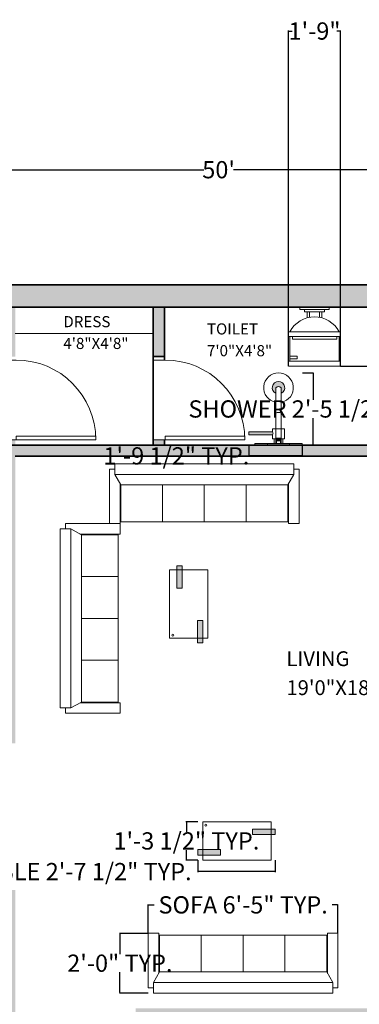
# Model space of a CAD drawing. Units: inches. Extents: x 1319 to 2030, y 219 to 1069.
# Tile 26 of 28: x 1589 to 1727, y 663 to 1063. Entities that reach past the tile are written whole.
import ezdxf

# ---------------------------------------------------------------- set-up
doc = ezdxf.new("R2010")
doc.units = ezdxf.units.IN
doc.header["$MEASUREMENT"] = 0
doc.layers.get('0').update_dxf_attribs({"color": 12})
for name, color, linetype, lineweight in [('A-ANNO-DIMS', 2, 'Continuous', 18), ('A-AREA-IDEN', 250, 'Continuous', 18), ('A-WALL-PATT', 252, 'Continuous', 13), ('C-PROP', 7, 'Continuous', 35), ('closet', 252, 'Continuous', 18), ('doors', 252, 'Continuous', 18), ('furniture', 250, 'Continuous', 18), ('PLUMBING FIXTURES', 252, 'Continuous', 18), ('walls', 250, 'Continuous', 35)]:
    doc.layers.add(name, color=color, linetype=linetype, lineweight=lineweight)
doc.styles.get("Standard").update_dxf_attribs({"font": 'arial.ttf'})
doc.dimstyles.get("Standard").update_dxf_attribs({"dimtxt": 7, "dimasz": 0.18, "dimexe": 0.18, "dimexo": 0.0625, "dimgap": 0.09, "dimtad": 0, "dimtih": 1, "dimtoh": 1, "dimzin": 0, "dimdsep": 46, "dimlunit": 3, "dimtxsty": 'Standard', "dimcen": 0.09, "dimadec": 0, "dimazin": 0, "dimtfac": 1, "dimtofl": 0, "dimtmove": 0, "dimatfit": 3, "dimfxl": 1, "dimtolj": 1, "dimtzin": 0, "dimarcsym": 0})

# ---------------------------------------------------------------- blocks, each defined once
blk = doc.blocks.new('*U2')
for p, q in [((0, 0), (0, -6)), ((40, 0), (40, -6))]:
    blk.add_line(p, q)
blk.add_lwpolyline([(0, 0), (0, 40), (1.75, 40), (1.75, 0)], close=True)
blk.add_arc((0, 0), 40, 0, 90)
blk = doc.blocks.new('FABRIC SOFA 4S')
at = {"layer": 'furniture'}
for p, q in [((0, -51), (0, 51)), ((6, 51), (0, 51)), ((3, 54), (34, 54)), ((3, 51), (3, 54)), ((6, -51), (6, 51)), ((12, 47.63), (6, 51)), ((34, 48), (34, 54)), ((11.14, 48), (34, 48)), ((33, 23.81), (12, 23.81)), ((33, 0), (12, 0)), ((33, -23.81), (12, -23.81)), ((6, -51), (12, -47.63)), ((11.54, -48), (34, -48)), ((34, -48), (34, -54)), ((6, -51), (0, -51)), ((3, -54), (3, -51)), ((3, -54), (34, -54))]:
    blk.add_line(p, q, dxfattribs=at)
blk.add_lwpolyline([(12, -47.63), (12, 47.63), (33, 47.63), (33, -47.63)], close=True, dxfattribs=at)
blk = doc.blocks.new('*U25')
for p, q in [((-10, 22), (-10, 12)), ((-10, 21), (-7, 21)), ((-7, 20), (-10, 20)), ((-7, 21), (-7, 20)), ((10, 12), (10, 22)), ((10.5, 12), (-10.5, 12)), ((-10.5, 10), (-10.5, 12)), ((9, 13), (-9, 13)), ((-9, 13), (-9, 12)), ((9, 12), (9, 13)), ((10.5, 12), (10.5, 10)), ((10.5, 10), (-10.5, 10)), ((-3, 4.4065), (-3, 2)), ((-2, 2), (-2, 4.1658)), ((2, 4.1658), (2, 2)), ((3, 2), (3, 4.4065)), ((4, 2), (-4, 2)), ((-4, 2), (-4, 1)), ((4, 1), (4, 2))]:
    blk.add_line(p, q)
for points in [[(10.5, 22), (10.5, 24), (-10.5, 24), (-10.5, 22)], [(6, 0), (6, 1), (-6, 1), (-6, 0)]]:
    blk.add_lwpolyline(points, close=True)
blk.add_arc((0, 15.3333), 11.3333, 208.0725, 331.9275)
blk = doc.blocks.new('O.H SHOWER-PL')
at = {"layer": 'PLUMBING FIXTURES'}
for points in [[(-1.84, 0), (-1.84, -0.25), (1.84, -0.25), (1.84, 0)], [(0.46, -8.72), (0.46, -9.67, -0.422337), (-0.46, -9.67), (-0.46, -8.72, 4.325472)]]:
    blk.add_hatch(color=256, dxfattribs=at).paths.add_polyline_path(points)
for p, q in [((-1.84, 0), (-1.84, -0.25)), ((1.84, 0), (-1.84, 0)), ((1.84, 0), (1.84, -0.25)), ((1.84, -0.25), (-1.84, -0.25)), ((-0.46, -0.25), (-0.46, -9.67)), ((0.46, -0.25), (0.46, -9.67))]:
    blk.add_line(p, q, dxfattribs=at)
for centre, radius, start, end in [((0, -4.48), 1.03, 243.53, 296.47), ((0, -9.67), 2.5, 100.61, 79.39), ((0, -9.67), 1.05, 116.0349, 63.9652), ((0, -9.22), 0.643, 224.2078, 315.7922)]:
    blk.add_arc(centre, radius, start, end, dxfattribs=at)
blk = doc.blocks.new('DIVERTER-PL')
at = {"layer": 'PLUMBING FIXTURES'}
for points in [[(4, 0), (-4, 0), (-4, -0.25), (4, -0.25)], [(0.38, -1.14), (0.38, -0.7), (-0.37, -0.7), (-0.37, -1.14)], [(1, -1.75, 0.30818), (1, -2.25), (5, -2.25), (5, -1.75)]]:
    blk.add_hatch(color=256, dxfattribs=at).paths.add_polyline_path(points)
for p, q in [((-4, 0), (-4, -0.25)), ((-4, 0), (4, 0)), ((4, 0), (4, -0.25)), ((-4, -0.25), (4, -0.25)), ((-4, -0.25), (4, -0.25)), ((-1, -1.05), (-0.37, -1.05)), ((-1, -1.05), (-1, -2.75)), ((-0.75, -0.25), (-0.75, -1.05)), ((-0.37, -0.7), (0.38, -0.7)), ((-0.37, -0.7), (-0.37, -1.14)), ((-0.37, -1.14), (0.38, -1.14)), ((-0.32, -0.7), (-0.32, -0.25)), ((0.32, -0.7), (0.32, -0.25)), ((0.38, -0.7), (0.38, -1.14)), ((0.38, -1.05), (1, -1.05)), ((0.75, -0.25), (0.75, -1.05)), ((1, -1.05), (1, -1.75)), ((-1, -2.75), (1, -2.75)), ((1, -2.25), (1, -2.75))]:
    blk.add_line(p, q, dxfattribs=at)
at = {"layer": 'PLUMBING FIXTURES', "ltscale": 12}
for p, q in [((1, -1.75), (5, -1.75)), ((1, -2.25), (5, -2.25)), ((5, -2.25), (5, -1.75))]:
    blk.add_line(p, q, dxfattribs=at)
at = {"layer": 'PLUMBING FIXTURES'}
blk.add_arc((1.37, -2), 0.444, 145.7435, 214.2565, dxfattribs=at)
blk = doc.blocks.new('A$C7F153053')
at = {"layer": 'PLUMBING FIXTURES', "xscale": -1, "rotation": 270}
for name in ['DIVERTER-PL', 'O.H SHOWER-PL']:
    blk.add_blockref(name, (12.17, 4), dxfattribs=at)
blk = doc.blocks.new('*D28')
at = {"layer": 'A-ANNO-DIMS', "color": 0, "lineweight": -2, "transparency": 16777216}
for p, q in [((1369.84, 1002.94), (1369.84, 1001.77)), ((1969.84, 1002.94), (1969.84, 1001.77)), ((1370.02, 1001.95), (1663.81, 1001.95)), ((1969.66, 1001.95), (1675.87, 1001.95))]:
    blk.add_line(p, q, dxfattribs=at)
at = {"layer": 'A-ANNO-DIMS', "color": 0, "transparency": 16777216}
for points in [[(1370.02, 1001.98), (1370.02, 1001.92), (1369.84, 1001.95)], [(1969.66, 1001.98), (1969.66, 1001.92), (1969.84, 1001.95)]]:
    blk.add_solid(points, dxfattribs=at)
at = {"layer": 'Defpoints', "color": 0, "transparency": 16777216}
for p in [(1369.84, 1003), (1969.84, 1003), (1969.84, 1001.95)]:
    blk.add_point(p, dxfattribs=at)
at = {"layer": 'A-ANNO-DIMS', "color": 0, "transparency": 16777216, "insert": (1669.84, 1001.95), "char_height": 7, "attachment_point": 5}
blk.add_mtext("\\A1;50'", dxfattribs=at)
blk = doc.blocks.new('TABLE-COCKTAIL')
h = blk.add_hatch(color=256)
h.dxf.hatch_style = 1
h.paths.add_polyline_path([(4.23, 29.31), (2.04, 29.31), (2.04, 22.19), (4.23, 22.19)])
h.paths.add_polyline_path([(4.23, 31.28), (2.04, 31.28), (2.04, 29.31), (4.23, 29.31)])
h.paths.add_polyline_path([(12.58, 9.09), (10.39, 9.09), (10.39, 1.62), (12.58, 1.62)])
h.paths.add_polyline_path([(12.58, 1.62), (10.39, 1.62), (10.39, 0), (12.58, 0)])
for p, q in [((0, 29.31), (0, 1.62)), ((15.53, 29.31), (0, 29.31)), ((2.04, 31.28), (4.23, 31.28)), ((2.04, 22.19), (2.04, 31.28)), ((4.23, 31.28), (4.23, 22.19)), ((15.53, 1.62), (15.53, 29.31)), ((4.23, 22.19), (2.04, 22.19)), ((10.39, 9.09), (12.58, 9.09)), ((10.39, 0), (10.39, 9.09)), ((12.58, 9.09), (12.58, 0)), ((0, 1.62), (15.53, 1.62)), ((12.58, 0), (10.39, 0))]:
    blk.add_line(p, q)
blk.add_circle((14.17, 28.1), 0.401)
blk = doc.blocks.new('*D36')
at = {"layer": 'A-ANNO-DIMS', "color": 0, "lineweight": -2, "transparency": 16777216}
for p, q in [((1641.31, 692.19), (1641.31, 703.85)), ((1641.49, 703.67), (1643.72, 703.67)), ((1718.11, 703.67), (1715.88, 703.67)), ((1718.29, 692.19), (1718.29, 703.85))]:
    blk.add_line(p, q, dxfattribs=at)
at = {"layer": 'A-ANNO-DIMS', "color": 0, "transparency": 16777216}
for points in [[(1641.49, 703.7), (1641.49, 703.64), (1641.31, 703.67)], [(1718.11, 703.7), (1718.11, 703.64), (1718.29, 703.67)]]:
    blk.add_solid(points, dxfattribs=at)
at = {"layer": 'Defpoints', "color": 0, "transparency": 16777216}
for p in [(1718.29, 703.67), (1641.31, 692.12), (1718.29, 692.12)]:
    blk.add_point(p, dxfattribs=at)
at = {"layer": 'A-ANNO-DIMS', "color": 0, "transparency": 16777216, "insert": (1679.8, 703.67), "char_height": 7, "attachment_point": 5}
blk.add_mtext('\\A1;SOFA 6\'-5" TYP.', dxfattribs=at)
blk = doc.blocks.new('*D37')
at = {"layer": 'A-ANNO-DIMS', "color": 0, "lineweight": -2, "transparency": 16777216}
for p, q in [((1641.25, 692.12), (1629.59, 692.12)), ((1629.77, 691.94), (1629.77, 683.67)), ((1629.77, 668.07), (1629.77, 676.34)), ((1641.25, 667.89), (1629.59, 667.89))]:
    blk.add_line(p, q, dxfattribs=at)
at = {"layer": 'A-ANNO-DIMS', "color": 0, "transparency": 16777216}
for points in [[(1629.74, 691.94), (1629.8, 691.94), (1629.77, 692.12)], [(1629.74, 668.07), (1629.8, 668.07), (1629.77, 667.89)]]:
    blk.add_solid(points, dxfattribs=at)
at = {"layer": 'Defpoints', "color": 0, "transparency": 16777216}
for p in [(1629.77, 692.12), (1641.31, 692.12), (1641.31, 667.89)]:
    blk.add_point(p, dxfattribs=at)
at = {"layer": 'A-ANNO-DIMS', "color": 0, "transparency": 16777216, "insert": (1629.77, 680.01), "char_height": 7, "attachment_point": 5}
blk.add_mtext('\\A1;2\'-0" TYP.', dxfattribs=at)
blk = doc.blocks.new('*D40')
at = {"layer": 'A-ANNO-DIMS', "color": 0, "lineweight": -2, "transparency": 16777216}
for p, q in [((1703.84, 919.51), (1708.35, 919.51)), ((1708.17, 919.33), (1708.17, 908.58)), ((1708.17, 890.41), (1708.17, 901.15)), ((1703.84, 890.23), (1708.35, 890.23))]:
    blk.add_line(p, q, dxfattribs=at)
at = {"layer": 'A-ANNO-DIMS', "color": 0, "transparency": 16777216}
for points in [[(1708.14, 919.33), (1708.2, 919.33), (1708.17, 919.51)], [(1708.14, 890.41), (1708.2, 890.41), (1708.17, 890.23)]]:
    blk.add_solid(points, dxfattribs=at)
at = {"layer": 'Defpoints', "color": 0, "transparency": 16777216}
for p in [(1703.78, 919.51), (1703.78, 890.23), (1708.17, 890.23)]:
    blk.add_point(p, dxfattribs=at)
at = {"layer": 'A-ANNO-DIMS', "color": 0, "transparency": 16777216, "insert": (1708.17, 904.87), "char_height": 7, "attachment_point": 5}
blk.add_mtext('\\A1;SHOWER 2\'-5 1/2" TYP.', dxfattribs=at)
blk = doc.blocks.new('*D41')
at = {"layer": 'A-ANNO-DIMS', "color": 0, "lineweight": -2, "transparency": 16777216}
for p, q in [((1682.12, 890.16), (1682.12, 885.66)), ((1703.78, 890.16), (1703.78, 885.66)), ((1682.12, 885.84), (1681.94, 885.84)), ((1703.6, 885.84), (1682.3, 885.84))]:
    blk.add_line(p, q, dxfattribs=at)
at = {"layer": 'A-ANNO-DIMS', "color": 0, "transparency": 16777216}
for points in [[(1682.3, 885.87), (1682.3, 885.81), (1682.12, 885.84)], [(1703.6, 885.87), (1703.6, 885.81), (1703.78, 885.84)]]:
    blk.add_solid(points, dxfattribs=at)
at = {"layer": 'Defpoints', "color": 0, "transparency": 16777216}
for p in [(1682.12, 890.23), (1703.78, 890.23), (1682.12, 885.84)]:
    blk.add_point(p, dxfattribs=at)
at = {"layer": 'A-ANNO-DIMS', "color": 0, "transparency": 16777216, "insert": (1652.69, 885.84), "char_height": 7, "attachment_point": 5}
blk.add_mtext('\\A1;1\'-9 1/2" TYP.', dxfattribs=at)
blk = doc.blocks.new('*D44')
at = {"layer": 'A-ANNO-DIMS', "color": 0, "lineweight": -2, "transparency": 16777216}
for p, q in [((1661.46, 721.8), (1661.46, 716.99)), ((1692.74, 721.8), (1692.74, 716.99)), ((1661.46, 717.17), (1661.28, 717.17)), ((1692.56, 717.17), (1661.64, 717.17))]:
    blk.add_line(p, q, dxfattribs=at)
at = {"layer": 'A-ANNO-DIMS', "color": 0, "transparency": 16777216}
for points in [[(1661.64, 717.2), (1661.64, 717.14), (1661.46, 717.17)], [(1692.56, 717.2), (1692.56, 717.14), (1692.74, 717.17)]]:
    blk.add_solid(points, dxfattribs=at)
at = {"layer": 'Defpoints', "color": 0, "transparency": 16777216}
for p in [(1661.46, 721.86), (1692.74, 721.86), (1661.46, 717.17)]:
    blk.add_point(p, dxfattribs=at)
at = {"layer": 'A-ANNO-DIMS', "color": 0, "transparency": 16777216, "insert": (1602.51, 717.17), "char_height": 7, "attachment_point": 5}
blk.add_mtext('\\A1;LOW TABLE 2\'-7 1/2" TYP.', dxfattribs=at)
blk = doc.blocks.new('*D45')
at = {"layer": 'A-ANNO-DIMS', "color": 0, "lineweight": -2, "transparency": 16777216}
for p, q in [((1661.4, 737.38), (1656.59, 737.38)), ((1656.77, 737.2), (1656.77, 733.33)), ((1656.77, 722.04), (1656.77, 725.91)), ((1661.4, 721.86), (1656.59, 721.86))]:
    blk.add_line(p, q, dxfattribs=at)
at = {"layer": 'A-ANNO-DIMS', "color": 0, "transparency": 16777216}
for points in [[(1656.74, 737.2), (1656.8, 737.2), (1656.77, 737.38)], [(1656.74, 722.04), (1656.8, 722.04), (1656.77, 721.86)]]:
    blk.add_solid(points, dxfattribs=at)
at = {"layer": 'Defpoints', "color": 0, "transparency": 16777216}
for p in [(1656.77, 737.38), (1661.46, 737.38), (1661.46, 721.86)]:
    blk.add_point(p, dxfattribs=at)
at = {"layer": 'A-ANNO-DIMS', "color": 0, "transparency": 16777216, "insert": (1656.77, 729.62), "char_height": 7, "attachment_point": 5}
blk.add_mtext('\\A1;1\'-3 1/2" TYP.', dxfattribs=at)
blk = doc.blocks.new('*D70')
at = {"layer": 'A-ANNO-DIMS', "color": 0, "lineweight": -2, "transparency": 16777216}
for p, q in [((1698.27, 922.29), (1698.27, 1058.4)), ((1698.45, 1058.22), (1699.7, 1058.22)), ((1719.09, 1058.22), (1717.83, 1058.22)), ((1719.27, 922.29), (1719.27, 1058.4))]:
    blk.add_line(p, q, dxfattribs=at)
at = {"layer": 'A-ANNO-DIMS', "color": 0, "transparency": 16777216}
for points in [[(1698.45, 1058.25), (1698.45, 1058.19), (1698.27, 1058.22)], [(1719.09, 1058.25), (1719.09, 1058.19), (1719.27, 1058.22)]]:
    blk.add_solid(points, dxfattribs=at)
at = {"layer": 'Defpoints', "color": 0, "transparency": 16777216}
for p in [(1719.27, 1058.22), (1698.27, 922.23), (1719.27, 922.23)]:
    blk.add_point(p, dxfattribs=at)
at = {"layer": 'A-ANNO-DIMS', "color": 0, "transparency": 16777216, "insert": (1708.77, 1058.22), "char_height": 7, "attachment_point": 5}
blk.add_mtext('\\A1;1\'-9"', dxfattribs=at)
blk = doc.blocks.new('*D71')
at = {"layer": 'A-ANNO-DIMS', "color": 0, "lineweight": -2, "transparency": 16777216}
for p, q in [((1714.83, 946.23), (2012.57, 946.23)), ((2012.39, 946.05), (2012.39, 937.89)), ((2012.39, 922.41), (2012.39, 930.56)), ((1719.33, 922.23), (2012.57, 922.23))]:
    blk.add_line(p, q, dxfattribs=at)
at = {"layer": 'A-ANNO-DIMS', "color": 0, "transparency": 16777216}
for points in [[(2012.36, 946.05), (2012.42, 946.05), (2012.39, 946.23)], [(2012.36, 922.41), (2012.42, 922.41), (2012.39, 922.23)]]:
    blk.add_solid(points, dxfattribs=at)
at = {"layer": 'Defpoints', "color": 0, "transparency": 16777216}
for p in [(1714.77, 946.23), (2012.39, 946.23), (1719.27, 922.23)]:
    blk.add_point(p, dxfattribs=at)
at = {"layer": 'A-ANNO-DIMS', "color": 0, "transparency": 16777216, "insert": (2012.39, 934.23), "char_height": 7, "attachment_point": 5}
blk.add_mtext('\\A1;2\'-0"', dxfattribs=at)

msp = doc.modelspace()

# ---------------------------------------------------------------- hatches: boundary and pattern name
at = {"layer": 'A-WALL-PATT'}
h = msp.add_hatch(color=256, dxfattribs=at)
h.dxf.hatch_style = 1
h.paths.add_polyline_path([(1378.843, 946.227), (1960.843, 946.227), (1960.843, 860.616), (1922.194, 860.616), (1922.194, 851.616), (1960.843, 851.616), (1960.843, 304.227), (1578.343, 304.227), (1578.343, 295.227), (1969.843, 295.227), (1969.843, 955.227), (1369.843, 955.227), (1369.843, 295.227), (1378.843, 295.227)])
h = msp.add_hatch(color=256, dxfattribs=at)
h.dxf.hatch_style = 1
h.paths.add_polyline_path([(1856.292, 860.616), (1812.343, 860.616), (1812.343, 851.616), (1812.343, 700.993), (1816.843, 700.993), (1816.843, 851.616), (1856.292, 851.616)])
h.paths.add_polyline_path([(1960.843, 663.616), (1812.343, 663.616), (1782.783, 663.616), (1782.783, 659.116), (1812.343, 659.116), (1960.843, 659.116)])
h.paths.add_polyline_path([(1857.424, 659.116), (1852.924, 659.116), (1852.924, 616.807), (1857.424, 616.807)])
h.paths.add_polyline_path([(1735.843, 661.727), (1731.843, 661.727), (1636.133, 661.727), (1636.133, 657.227), (1731.343, 657.227), (1731.343, 481.227), (1618.616, 481.227), (1618.616, 472.227), (1639.343, 472.227), (1639.343, 384.227), (1627.044, 384.227), (1627.044, 375.227), (1648.343, 375.227), (1648.343, 384.227), (1648.343, 472.227), (1750.706, 472.227), (1750.706, 481.227), (1735.843, 481.227), (1735.843, 657.727)])
h.paths.add_polyline_path([(1587.343, 481.227), (1578.343, 481.227), (1578.343, 375.227), (1597.622, 375.227), (1597.622, 384.227), (1587.343, 384.227)])
h.paths.add_polyline_path([(1769.593, 384.227), (1693.482, 384.227), (1693.482, 375.227), (1769.593, 375.227)])
h.paths.add_polyline_path([(1775.828, 481.227), (1765.831, 481.227), (1765.831, 472.227), (1775.828, 472.227)])
h.paths.add_polyline_path([(1824.625, 481.227), (1820.343, 481.227), (1820.343, 476.727), (1824.625, 476.727), (1824.625, 477.545)], flags=0)
h.paths.add_polyline_path([(1896.843, 481.227), (1852.26, 481.227), (1852.26, 476.727), (1892.343, 476.727), (1892.343, 384.227), (1881.742, 384.227), (1881.742, 375.227), (1913.435, 375.227), (1913.435, 384.227), (1896.843, 384.227)])
h.paths.add_polyline_path([(1960.843, 481.227), (1931.341, 481.227), (1931.341, 476.727), (1960.843, 476.727)])
h.paths.add_polyline_path([(1736.343, 918.227), (1731.843, 918.227), (1731.843, 890.227), (1582.843, 890.227), (1582.843, 781.727), (1582.843, 769.171), (1587.343, 769.171), (1587.343, 781.727), (1587.343, 885.727), (1731.843, 885.727), (1731.843, 851.616), (1736.343, 851.616), (1736.343, 890.227)])
h.paths.add_polyline_path([(1781.022, 860.616), (1773.021, 860.616, -0.0322281), (1773.289, 856.464), (1773.289, 851.616), (1781.022, 851.616)])
h.paths.add_polyline_path([(1587.343, 946.227), (1582.843, 946.227), (1582.843, 926.136), (1587.343, 926.136)])
h.paths.add_polyline_path([(1647.843, 946.227), (1643.343, 946.227), (1643.343, 926.136), (1647.843, 926.136)])
h.paths.add_polyline_path([(1543.343, 786.227), (1429.843, 786.227), (1429.843, 757.555), (1434.343, 757.555), (1438.843, 757.555), (1438.843, 781.727), (1543.343, 781.727)])
h.paths.add_polyline_path([(1543.343, 781.727), (1538.843, 781.727), (1538.843, 709.727), (1534.597, 709.727), (1534.597, 705.227), (1543.343, 705.227), (1543.343, 709.727)])
h.paths.add_polyline_path([(1499.955, 709.727), (1438.843, 709.727), (1438.843, 734.463), (1429.843, 734.463), (1429.843, 552.227), (1470.241, 552.227), (1470.241, 561.227), (1438.843, 561.227), (1438.843, 705.227), (1499.955, 705.227)])
h.paths.add_polyline_path([(1587.343, 709.727), (1582.843, 709.727), (1582.843, 561.227), (1543.433, 561.227), (1543.433, 552.227), (1587.343, 552.227)])
h.paths.add_polyline_path([(1546.835, 709.727), (1543.343, 709.727), (1543.343, 705.227), (1546.835, 705.227)])
h.paths.add_polyline_path([(1582.843, 709.727), (1579.15, 709.727), (1579.15, 705.227), (1582.843, 705.227)], flags=17)
h.paths.add_polyline_path([(1548.368, 786.227), (1543.343, 786.227), (1543.343, 781.727), (1548.368, 781.727)])
h.paths.add_polyline_path([(1582.843, 786.227), (1580.683, 786.227), (1580.683, 781.727), (1582.843, 781.727)])
h.paths.add_polyline_path([(1587.343, 892.402), (1582.843, 892.402), (1582.843, 890.227), (1587.343, 890.227)], flags=17)
h.paths.add_polyline_path([(1647.843, 892.402), (1643.343, 892.402), (1643.343, 890.227), (1647.843, 890.227)], flags=17)
h.paths.add_polyline_path([(1740.974, 856.464), (1740.974, 860.616), (1736.343, 860.616), (1736.343, 851.616), (1740.974, 851.616)])
h.paths.add_polyline_path([(1853.989, 384.227), (1820.343, 384.227), (1820.343, 402.924), (1815.843, 402.924), (1815.843, 375.227), (1853.989, 375.227)])
h.paths.add_polyline_path([(1892.343, 436.227), (1820.343, 436.227), (1820.343, 481.227), (1815.843, 481.227), (1815.843, 431.727), (1892.343, 431.727)])
h.paths.add_polyline_path([(1849.175, 481.227), (1824.625, 481.227), (1824.625, 477.545), (1825.699, 477.545), (1825.699, 453.018, 0.4014527), (1849.175, 477.545)], flags=0)
h.paths.add_polyline_path([(1960.843, 384.227), (1941.188, 384.227), (1941.188, 375.227), (1960.843, 375.227)])
h.paths.add_polyline_path([(1902.267, 481.227), (1896.843, 481.227), (1896.843, 476.727), (1902.267, 476.727), (1902.267, 477.44)], flags=0)

# ---------------------------------------------------------------- linework, layer by layer
at = {"layer": 'C-PROP'}
msp.add_line((1369.843, 955.227), (1969.843, 955.227), dxfattribs=at)
at = {"layer": 'closet'}
msp.add_line((1587.343, 935.472), (1643.343, 935.472), dxfattribs=at)
at = {"layer": 'walls'}
for p, q in [((1378.843, 946.227), (1960.843, 946.227)), ((1643.343, 890.227), (1643.343, 946.227)), ((1647.843, 924.716), (1647.843, 946.227)), ((1643.343, 926.136), (1647.843, 926.136)), ((1647.843, 890.227), (1647.843, 892.402)), ((1582.843, 890.227), (1731.843, 890.227)), ((1587.343, 885.727), (1731.843, 885.727))]:
    msp.add_line(p, q, dxfattribs=at)

# ---------------------------------------------------------------- block references
at = {"layer": 'doors', "xscale": -0.8078659498341503, "yscale": 0.8078659498341503, "zscale": 0.8078659498341503, "rotation": 270}
for p in [(1587.69, 892.402), (1648.19, 892.402)]:
    msp.add_blockref('*U2', p, dxfattribs=at)
at = {"layer": 'furniture', "yscale": 0.7127038693416449, "zscale": 0.7127038693416449, "rotation": 270}
for p, xscale in [((1664.047, 882.622), 0.7127038693416449), ((1679.8, 667.892), -0.7127038693416449)]:
    msp.add_blockref('FABRIC SOFA 4S', p, dxfattribs=dict(at, xscale=xscale))
at = {"layer": 'furniture', "xscale": 0.7127038693416449, "yscale": 0.7127038693416449, "zscale": 0.7127038693416449}
msp.add_blockref('FABRIC SOFA 4S', (1605.606, 819.904), dxfattribs=at)
at = {"layer": 'furniture'}
for p, rotation in [((1665.489, 841.233), 180), ((1692.741, 721.858), 90.00000000000365)]:
    msp.add_blockref('TABLE-COCKTAIL', p, dxfattribs=dict(at, rotation=rotation))
at = {"layer": 'PLUMBING FIXTURES', "xscale": -1, "rotation": 180}
msp.add_blockref('*U25', (1708.765, 946.227), dxfattribs=at)
at = {"layer": 'PLUMBING FIXTURES', "xscale": -2.406230429091579, "yscale": 2.406230429091579, "zscale": 2.406230429091579, "rotation": 90}
msp.add_blockref('A$C7F153053', (1703.778, 919.501), dxfattribs=at)

# ---------------------------------------------------------------- texts
at = {"layer": 'A-AREA-IDEN'}
for s, height, p in [('DRESS', 4.5146, (1606.812, 938.031)), ('TOILET', 4.5146, (1665.108, 935.092)), ('4\'8"X4\'8"', 4.5146, (1606.812, 929.207)), ('7\'0"X4\'8"', 4.5146, (1665.108, 926.268)), ('LIVING', 6.0112, (1697.378, 800.537)), ('19\'0"X18\'8"', 6.01124, (1697.378, 788.788))]:
    msp.add_text(s, height=height, dxfattribs=at).set_placement(p)

# ---------------------------------------------------------------- dimensions: what is measured, and where the dimension line sits
at = {"layer": 'A-ANNO-DIMS'}
for base, p1, p2, override, picture, middle in [((1719.265, 1058.218), (1698.265, 922.227), (1719.265, 922.227), {"dimdec": 1, "dimlfac": 1, "dimrnd": 0, "dimzin": 1, "dimdsep": 46, "dimlunit": 4, "dimfrac": 2}, '*D70', (1708.765, 1058.218)), ((1969.843, 1001.954), (1369.843, 1003), (1969.843, 1003), {"dimclrd": 0, "dimclre": 0, "dimclrt": 0}, '*D28', (1669.843, 1001.954))]:
    dim = msp.add_linear_dim(base=base, p1=p1, p2=p2, dimstyle='Standard', override=override, dxfattribs=at)
    dim.commit()
    dim.dimension.update_dxf_attribs({"geometry": picture, "text_midpoint": middle})
dim = msp.add_linear_dim(base=(2012.394, 946.227), p1=(1719.265, 922.227), p2=(1714.765, 946.227), angle=90, dimstyle='Standard', override={"dimdec": 1, "dimlfac": 1, "dimrnd": 0, "dimzin": 1, "dimdsep": 46, "dimlunit": 4, "dimfrac": 2}, dxfattribs=at)
dim.commit()
dim.dimension.update_dxf_attribs({"geometry": '*D71', "text_midpoint": (2012.394, 934.227)})
for base, p1, p2, angle, text, picture, middle in [((1708.17, 890.227), (1703.778, 919.506), (1703.778, 890.227), 270, 'SHOWER <> TYP.', '*D40', (1708.17, 904.867)), ((1682.122, 885.835), (1703.778, 890.227), (1682.122, 890.227), 180, '<> TYP.', '*D41', (1652.692, 885.835)), ((1661.464, 717.166), (1692.742, 721.858), (1661.464, 721.858), 180, 'LOW TABLE <> TYP.', '*D44', (1602.515, 717.166)), ((1656.772, 737.383), (1661.464, 721.858), (1661.464, 737.383), 90, '<> TYP.', '*D45', (1656.772, 729.62)), ((1629.768, 692.124), (1641.314, 667.892), (1641.314, 692.124), 90, '<> TYP.', '*D37', (1629.768, 680.008))]:
    dim = msp.add_linear_dim(base=base, p1=p1, p2=p2, angle=angle, text=text, dimstyle='Standard', override={"dimdec": 1, "dimlfac": 1, "dimrnd": 0, "dimzin": 1, "dimdsep": 46, "dimlunit": 4, "dimfrac": 2}, dxfattribs=at)
    dim.commit()
    dim.dimension.update_dxf_attribs({"geometry": picture, "text_midpoint": middle})
dim = msp.add_linear_dim(base=(1718.286, 703.67), p1=(1641.314, 692.124), p2=(1718.286, 692.124), text='SOFA <> TYP.', dimstyle='Standard', override={"dimdec": 1, "dimlfac": 1, "dimrnd": 0, "dimzin": 1, "dimdsep": 46, "dimlunit": 4, "dimfrac": 2}, dxfattribs=at)
dim.commit()
dim.dimension.update_dxf_attribs({"geometry": '*D36', "text_midpoint": (1679.8, 703.67)})

doc.saveas('drawing.dxf')
